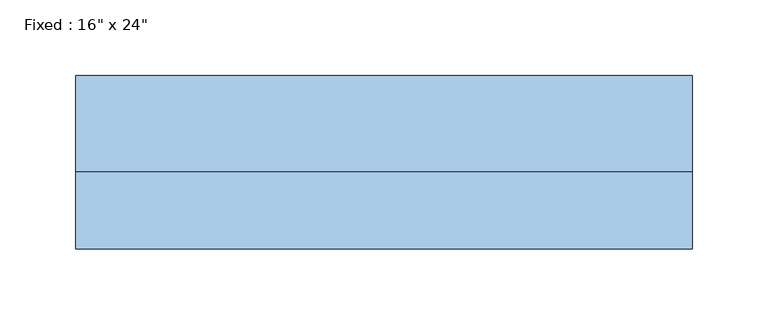
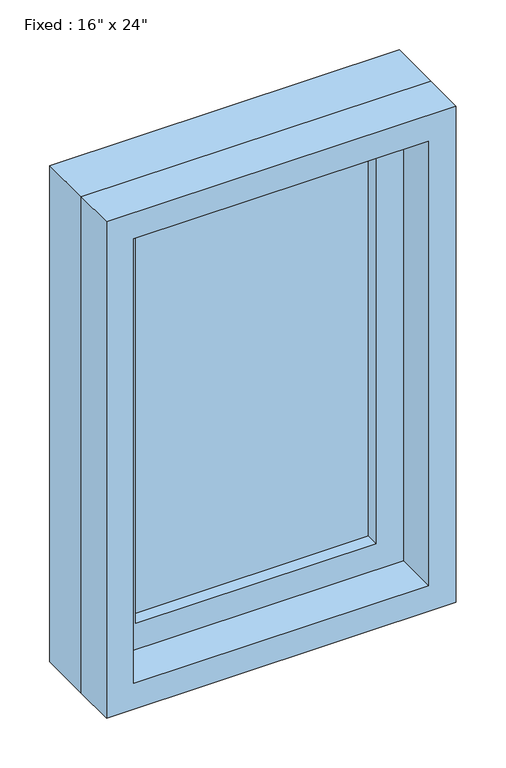
"""IFC4 building model written with IfcOpenShell, lengths in millimetres: window geometry."""

from ifc_helpers import new_model, si_unit, frame, origin, place, context, project, spatial, polyline, outline, extrude, source, transform, mapped, element, save


def window_a10b4202(model_context):
    return source(origin(), model_context, "Body", "SweptSolid", [
        extrude(outline(polyline([(101.6, 9.525), (-177.8, 9.525), (-177.8, 22.225), (101.6, 22.225), (101.6, 9.525)])), frame((0.0, 0.0, 977.9), z_axis=(0.0, 0.0, 1.0), x_axis=(1.0, 0.0, 0.0)), (0.0, 0.0, 1.0), 482.6),
        extrude(outline(polyline([(1504.95, -222.25), (933.45, -222.25), (933.45, 146.05), (1504.95, 146.05), (1504.95, -222.25)]), holes=[polyline([(1460.5, -177.8), (1460.5, 101.6), (977.9, 101.6), (977.9, -177.8), (1460.5, -177.8)])]), frame((0.0, -6.35, 0.0), z_axis=(0.0, 1.0, 0.0), x_axis=(0.0, 0.0, 1.0)), (0.0, 0.0, 1.0), 44.45),
        extrude(outline(polyline([(1524.0, -241.3), (914.4, -241.3), (914.4, 165.1), (1524.0, 165.1), (1524.0, -241.3)]), holes=[polyline([(1492.25, -209.55), (1492.25, 133.35), (946.15, 133.35), (946.15, -209.55), (1492.25, -209.55)])]), frame((0.0, -57.15, 0.0), z_axis=(0.0, 1.0, 0.0), x_axis=(0.0, 0.0, 1.0)), (0.0, 0.0, 1.0), 50.8),
        extrude(outline(polyline([(1524.0, 165.1), (1524.0, -241.3), (914.4, -241.3), (914.4, 165.1), (1524.0, 165.1)]), holes=[polyline([(1504.95, 146.05), (933.45, 146.05), (933.45, -222.25), (1504.95, -222.25), (1504.95, 146.05)])]), frame((0.0, -6.35, 0.0), z_axis=(0.0, 1.0, 0.0), x_axis=(0.0, 0.0, 1.0)), (0.0, 0.0, 1.0), 63.5),
    ])


if __name__ == "__main__":
    model = new_model("IFC4")
    model_context = context("Model", 3, world=origin())
    ifc_project = project(units=[si_unit("LENGTHUNIT", "METRE", prefix="MILLI")], contexts=[model_context])
    site = spatial("IfcSite", under=ifc_project)
    building = spatial("IfcBuilding", under=site)
    placement = place(None, origin())
    window_shape = window_a10b4202(model_context)
    element("IfcWindow", 1, ObjectType="Fixed : 16\" x 24\"", at=placement, inside=building, context=model_context, shape_type="MappedRepresentation", body=[
        mapped(window_shape, transform((0.0, 0.0, 0.0), x_axis=(1.0, 0.0, 0.0), y_axis=(0.0, 1.0, 0.0), z_axis=(0.0, 0.0, 1.0))),
    ])
    save(model, "model.ifc")

# Revit data of these elements
# Type "Fixed : 16\" x 24\""
#   Type Mark = "4"
#   Construction Type Id = "GSP4R"
#   Assembly Code = "B2020100"
#   Analytic Construction = "1/8 in Pilkington single glazing"
#   Visual Light Transmittance = 0.9
#   Solar Heat Gain Coefficient = 0.78
#   Heat Transfer Coefficient (U) = 0.6496 BTU/(h·ft²·°F)
#   Height = 2' - 0"
#   Default Sill Height = 3' - 0"
#   Width = 1' - 4"
#   Window Inset = 0' - 0 3/4"
#   Define Thermal Properties by = 1
#   Define Thermal Properties by = 1
#   Glass Pane Material = Glass
#   Sash Material = Sash
#   Wall Closure = (empty or 0)
# Element 1 (IfcWindow, "Fixed : 16\" x 24\"")
#   Materials on its faces: "Sash", "Glass"
# Materials
#   "Glass": class "Glass", colour RGB 0 128 192, transparency 0.75, Description = "Soda Lime Glass", Cost = 0
#   "Sash": class "Wood", colour RGB 224 178 126, transparency 0, Cost = 0
